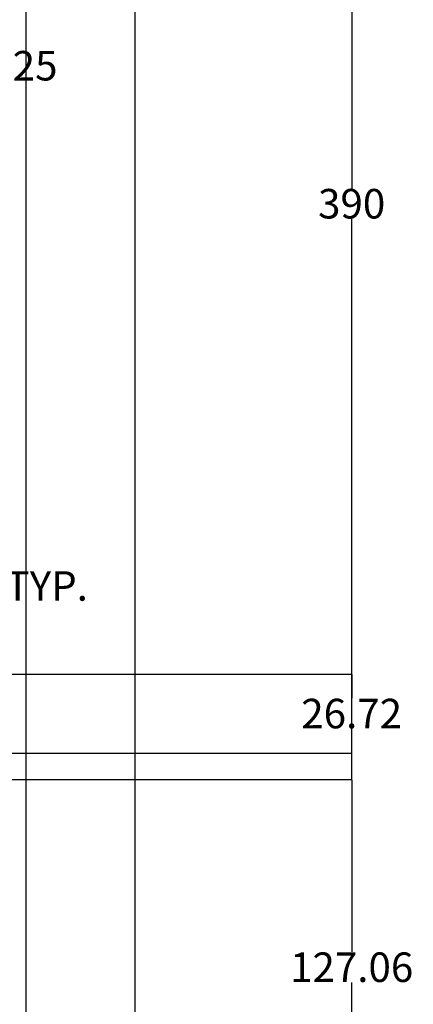
# Model space of a CAD drawing. Units: inches. Extents: x 300 to 1007, y 2 to 1069.
# Tile 11 of 12: x 862 to 995, y 533 to 867. Entities that reach past the tile are written whole.
import ezdxf

# ---------------------------------------------------------------- set-up
doc = ezdxf.new("R2010")
doc.units = ezdxf.units.IN
doc.header["$MEASUREMENT"] = 0
doc.layers.add('A-ANNO-DIMS', color=2, linetype='Continuous', lineweight=18)
doc.styles.get("Standard").update_dxf_attribs({"font": 'arial.ttf'})
doc.dimstyles.get("Standard").update_dxf_attribs({"dimtxt": 10, "dimasz": 0.18, "dimexe": 0.18, "dimexo": 0.0625, "dimgap": 0.09, "dimtad": 0, "dimtih": 1, "dimtoh": 1, "dimdec": 0, "dimzin": 0, "dimdsep": 46, "dimlunit": 3, "dimtxsty": 'Standard', "dimcen": 0.09, "dimadec": 0, "dimazin": 0, "dimtfac": 1, "dimtdec": 0, "dimtofl": 0, "dimtmove": 0, "dimatfit": 3, "dimfxl": 1, "dimtolj": 1, "dimtzin": 0, "dimarcsym": 0})

# ---------------------------------------------------------------- blocks, each defined once
blk = doc.blocks.new('*D23')
at = {"layer": 'A-ANNO-DIMS', "color": 0, "lineweight": -2, "transparency": 16777216}
for p, q in [((797.11, 833.59), (814.61, 850.93)), ((817.34, 848.44), (814.61, 851.18)), ((814.74, 851.06), (814.87, 851.18)), ((814.87, 851.18), (815.05, 851.18)), ((799.58, 830.84), (796.86, 833.59))]:
    blk.add_line(p, q, dxfattribs=at)
at = {"layer": 'A-ANNO-DIMS', "color": 0, "transparency": 16777216}
for points in [[(814.59, 850.95), (814.63, 850.91), (814.74, 851.06)], [(797.09, 833.61), (797.13, 833.57), (796.98, 833.46)]]:
    blk.add_solid(points, dxfattribs=at)
at = {"layer": 'Defpoints', "color": 0, "transparency": 16777216}
for p in [(814.74, 851.06), (817.38, 848.39), (799.62, 830.8)]:
    blk.add_point(p, dxfattribs=at)
at = {"layer": 'A-ANNO-DIMS', "color": 0, "transparency": 16777216, "insert": (845.95, 851.18), "char_height": 10, "attachment_point": 5}
blk.add_mtext('\\A1;CHAIR 25', dxfattribs=at)
blk = doc.blocks.new('*D71')
at = {"layer": 'A-ANNO-DIMS', "color": 0, "lineweight": -2, "transparency": 16777216}
for p, q in [((768.17, 674), (768.17, 675.21)), ((768.35, 675.03), (775.25, 675.03)), ((775.43, 674), (775.43, 675.21)), ((775.43, 675.03), (775.61, 675.03))]:
    blk.add_line(p, q, dxfattribs=at)
at = {"layer": 'A-ANNO-DIMS', "color": 0, "transparency": 16777216}
for points in [[(768.35, 675.06), (768.35, 675), (768.17, 675.03)], [(775.25, 675.06), (775.25, 675), (775.43, 675.03)]]:
    blk.add_solid(points, dxfattribs=at)
at = {"layer": 'Defpoints', "color": 0, "transparency": 16777216}
for p in [(768.17, 673.94), (775.43, 675.03), (775.43, 673.94)]:
    blk.add_point(p, dxfattribs=at)
at = {"layer": 'A-ANNO-DIMS', "color": 0, "transparency": 16777216, "insert": (832.37, 675.03), "char_height": 10, "attachment_point": 5}
blk.add_mtext('\\A1;HOB RING 7 TYP.', dxfattribs=at)
blk = doc.blocks.new('*D77')
at = {"layer": 'A-ANNO-DIMS', "color": 0, "lineweight": -2, "transparency": 16777216}
for p, q in [((841.89, 609.45), (974.48, 609.45)), ((974.3, 609.27), (974.3, 551.11)), ((974.3, 482.56), (974.3, 540.72)), ((850.89, 482.38), (974.48, 482.38))]:
    blk.add_line(p, q, dxfattribs=at)
at = {"layer": 'A-ANNO-DIMS', "color": 0, "transparency": 16777216}
for points in [[(974.27, 609.27), (974.33, 609.27), (974.3, 609.45)], [(974.27, 482.56), (974.33, 482.56), (974.3, 482.38)]]:
    blk.add_solid(points, dxfattribs=at)
at = {"layer": 'Defpoints', "color": 0, "transparency": 16777216}
for p in [(841.83, 609.45), (974.3, 609.45), (850.83, 482.38)]:
    blk.add_point(p, dxfattribs=at)
at = {"layer": 'A-ANNO-DIMS', "color": 0, "transparency": 16777216, "insert": (974.3, 545.92), "char_height": 10, "attachment_point": 5}
blk.add_mtext('\\A1;127.06', dxfattribs=at)
blk = doc.blocks.new('*D78')
at = {"layer": 'A-ANNO-DIMS', "color": 0, "lineweight": -2, "transparency": 16777216}
for p, q in [((850.89, 999.45), (974.48, 999.45)), ((974.3, 999.27), (974.3, 809.65)), ((974.3, 609.63), (974.3, 799.25)), ((841.89, 609.45), (974.48, 609.45))]:
    blk.add_line(p, q, dxfattribs=at)
at = {"layer": 'A-ANNO-DIMS', "color": 0, "transparency": 16777216}
for points in [[(974.27, 999.27), (974.33, 999.27), (974.3, 999.45)], [(974.27, 609.63), (974.33, 609.63), (974.3, 609.45)]]:
    blk.add_solid(points, dxfattribs=at)
at = {"layer": 'Defpoints', "color": 0, "transparency": 16777216}
for p in [(850.83, 999.45), (974.3, 999.45), (841.83, 609.45)]:
    blk.add_point(p, dxfattribs=at)
at = {"layer": 'A-ANNO-DIMS', "color": 0, "transparency": 16777216, "insert": (974.3, 804.45), "char_height": 10, "attachment_point": 5}
blk.add_mtext('\\A1;390', dxfattribs=at)
blk = doc.blocks.new('*D83')
at = {"layer": 'A-ANNO-DIMS', "color": 0, "lineweight": -2, "transparency": 16777216}
for p, q in [((763.96, 645.17), (974.48, 645.17)), ((974.3, 644.99), (974.3, 637)), ((974.3, 618.63), (974.3, 626.61)), ((779.89, 618.45), (974.48, 618.45))]:
    blk.add_line(p, q, dxfattribs=at)
at = {"layer": 'A-ANNO-DIMS', "color": 0, "transparency": 16777216}
for points in [[(974.27, 644.99), (974.33, 644.99), (974.3, 645.17)], [(974.27, 618.63), (974.33, 618.63), (974.3, 618.45)]]:
    blk.add_solid(points, dxfattribs=at)
at = {"layer": 'Defpoints', "color": 0, "transparency": 16777216}
for p in [(763.9, 645.17), (974.3, 645.17), (779.83, 618.45)]:
    blk.add_point(p, dxfattribs=at)
at = {"layer": 'A-ANNO-DIMS', "color": 0, "transparency": 16777216, "insert": (974.3, 631.81), "char_height": 10, "attachment_point": 5}
blk.add_mtext('\\A1;26.72', dxfattribs=at)
blk = doc.blocks.new('*D84')
at = {"layer": 'A-ANNO-DIMS', "color": 0, "lineweight": -2, "transparency": 16777216}
for p, q in [((864.25, 225.89), (864.25, 1063.03)), ((864.43, 1062.85), (865.73, 1062.85)), ((900.94, 1062.85), (899.65, 1062.85)), ((901.12, 225.89), (901.12, 1063.03))]:
    blk.add_line(p, q, dxfattribs=at)
at = {"layer": 'A-ANNO-DIMS', "color": 0, "transparency": 16777216}
for points in [[(864.43, 1062.88), (864.43, 1062.82), (864.25, 1062.85)], [(900.94, 1062.88), (900.94, 1062.82), (901.12, 1062.85)]]:
    blk.add_solid(points, dxfattribs=at)
at = {"layer": 'Defpoints', "color": 0, "transparency": 16777216}
for p in [(901.12, 1062.85), (864.25, 225.83), (901.12, 225.83)]:
    blk.add_point(p, dxfattribs=at)
at = {"layer": 'A-ANNO-DIMS', "color": 0, "transparency": 16777216, "insert": (882.69, 1062.85), "char_height": 10, "attachment_point": 5}
blk.add_mtext('\\A1;36.87', dxfattribs=at)
blk = doc.blocks.new('*D86')
at = {"layer": 'A-ANNO-DIMS', "color": 0, "lineweight": -2, "transparency": 16777216}
for p, q in [((805.95, 235.15), (805.95, 1063.03)), ((806.13, 1062.85), (822.02, 1062.85)), ((864.07, 1062.85), (848.18, 1062.85)), ((864.25, 235.15), (864.25, 1063.03))]:
    blk.add_line(p, q, dxfattribs=at)
at = {"layer": 'A-ANNO-DIMS', "color": 0, "transparency": 16777216}
for points in [[(806.13, 1062.88), (806.13, 1062.82), (805.95, 1062.85)], [(864.07, 1062.88), (864.07, 1062.82), (864.25, 1062.85)]]:
    blk.add_solid(points, dxfattribs=at)
at = {"layer": 'Defpoints', "color": 0, "transparency": 16777216}
for p in [(864.25, 1062.85), (805.95, 235.08), (864.25, 235.08)]:
    blk.add_point(p, dxfattribs=at)
at = {"layer": 'A-ANNO-DIMS', "color": 0, "transparency": 16777216, "insert": (835.1, 1062.85), "char_height": 10, "attachment_point": 5}
blk.add_mtext('\\A1;58.3', dxfattribs=at)

msp = doc.modelspace()

# ---------------------------------------------------------------- dimensions: what is measured, and where the dimension line sits
at = {"layer": 'A-ANNO-DIMS'}
for base, p1, p2, override, picture, middle in [((864.2528, 1062.8469), (805.95, 235.0834), (864.2528, 235.0834), {"dimdec": 1, "dimlfac": 1, "dimrnd": 0, "dimzin": 0, "dimdsep": 46, "dimlunit": 2}, '*D86', (835.1014, 1062.8469)), ((901.1217, 1062.8469), (864.2528, 225.8264), (901.1217, 225.8264), {"dimdec": 2, "dimlfac": 1, "dimrnd": 0, "dimzin": 0, "dimdsep": 46, "dimlunit": 2}, '*D84', (882.6872, 1062.8469))]:
    dim = msp.add_linear_dim(base=base, p1=p1, p2=p2, dimstyle='Standard', override=override, dxfattribs=at)
    dim.commit()
    dim.dimension.update_dxf_attribs({"geometry": picture, "text_midpoint": middle})
for base, p1, p2, override, picture, middle in [((974.3023, 999.4468), (841.8267, 609.4468), (850.8267, 999.4468), {"dimdec": 0, "dimlfac": 1, "dimrnd": 0, "dimzin": 0, "dimdsep": 46, "dimlunit": 2}, '*D78', (974.3023, 804.4468)), ((974.3023, 645.167), (779.8267, 618.4468), (763.9001, 645.167), {"dimdec": 2, "dimlfac": 1, "dimrnd": 0, "dimzin": 0, "dimdsep": 46, "dimlunit": 2}, '*D83', (974.3023, 631.8069)), ((974.3023, 609.4468), (850.8267, 482.3847), (841.8267, 609.4468), {"dimdec": 2, "dimlfac": 1, "dimrnd": 0, "dimzin": 0, "dimdsep": 46, "dimlunit": 2}, '*D77', (974.3023, 545.9158))]:
    dim = msp.add_linear_dim(base=base, p1=p1, p2=p2, angle=90, dimstyle='Standard', override=override, dxfattribs=at)
    dim.commit()
    dim.dimension.update_dxf_attribs({"geometry": picture, "text_midpoint": middle})
dim = msp.add_linear_dim(base=(814.7415, 851.0564), p1=(799.6215, 830.8005), p2=(817.3803, 848.3926), angle=44.729737, text='CHAIR <>', dimstyle='Standard', override={"dimdec": 0, "dimlfac": 1, "dimrnd": 0, "dimzin": 0, "dimdsep": 46, "dimlunit": 2}, dxfattribs=at)
dim.commit()
dim.dimension.update_dxf_attribs({"geometry": '*D23', "text_midpoint": (845.9545, 851.1831)})
dim = msp.add_linear_dim(base=(775.4308, 675.0284), p1=(768.1736, 673.9399), p2=(775.4308, 673.9399), text='HOB RING <> TYP.', dimstyle='Standard', override={"dimdec": 0, "dimlfac": 1, "dimrnd": 0, "dimzin": 0, "dimdsep": 46, "dimlunit": 2}, dxfattribs=at)
dim.commit()
dim.dimension.update_dxf_attribs({"geometry": '*D71', "text_midpoint": (832.3652, 675.0284)})

doc.saveas('drawing.dxf')
